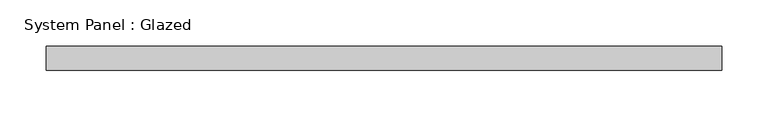
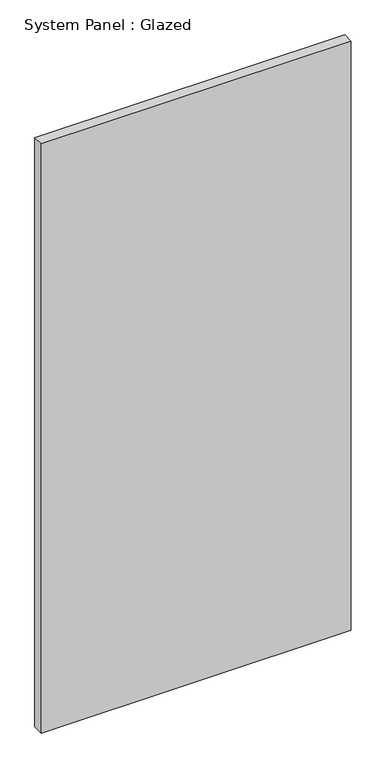
"""IFC4 building model written with IfcOpenShell, lengths in millimetres: plate geometry, System Panel : Glazed."""

from ifc_helpers import new_model, si_unit, origin, origin_with_axes, place, context, project, spatial, polyline, outline, extrude, source, transform, mapped, element, save


def system_panel_glazed_135d4218(model_context):
    return source(origin(), model_context, "Body", "SweptSolid", [
        extrude(outline(polyline([(363.0083333, 19.05), (-363.0083333, 19.05), (-363.0083333, 44.45), (363.0083333, 44.45), (363.0083333, 19.05)])), origin_with_axes(), (0.0, 0.0, 1.0), 1457.3599864),
    ])


if __name__ == "__main__":
    model = new_model("IFC4")
    model_context = context("Model", 3, world=origin())
    ifc_project = project(units=[si_unit("LENGTHUNIT", "METRE", prefix="MILLI")], contexts=[model_context])
    site = spatial("IfcSite", under=ifc_project)
    building = spatial("IfcBuilding", under=site)
    placement = place(None, origin())
    system_panel_glazed_shape = system_panel_glazed_135d4218(model_context)
    element("IfcPlate", 1, ObjectType="System Panel : Glazed", at=placement, inside=building, context=model_context, shape_type="MappedRepresentation", body=[
        mapped(system_panel_glazed_shape, transform((0.0, 0.0, 0.0), x_axis=(1.0, 0.0, 0.0), y_axis=(0.0, 1.0, 0.0), z_axis=(0.0, 0.0, 1.0))),
    ])
    save(model, "model.ifc")

# Revit data of these elements
# Type "System Panel : Glazed"
#   Construction Type Id = "GSP4R"
#   Analytic Construction = "1/8 in Pilkington single glazing"
#   Visual Light Transmittance = 0.9
#   Solar Heat Gain Coefficient = 0.86
#   Heat Transfer Coefficient (U) = 1.18115 BTU/(h·ft²·°F)
#   Define Thermal Properties by = 1
# Element 1 (IfcPlate, "System Panel : Glazed")
#   Materials on its faces: "Glass"
# Materials
#   "Glass": class "Glass", colour RGB 0 128 192, transparency 0.75, Description = "Soda Lime Glass", Cost = 0
